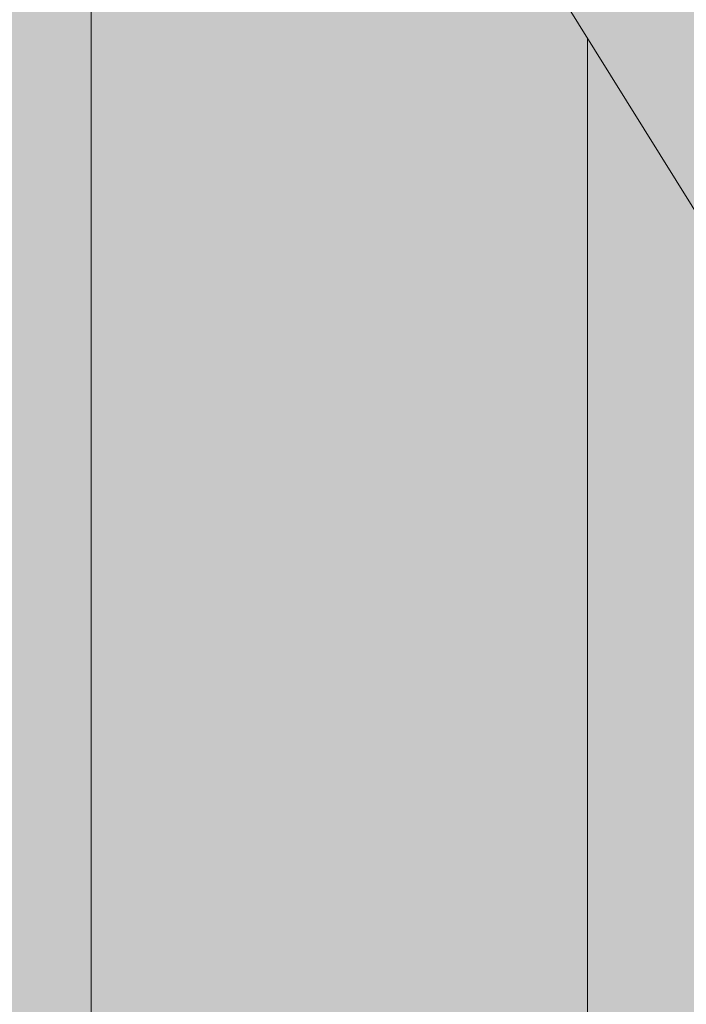
# Model space of a CAD drawing. Units: millimetres. Extents: x 11032 to 26788, y 3406 to 24505.
# Tile 48 of 78: x 15652 to 15719, y 16177 to 16276. Entities that reach past the tile are written whole.
import ezdxf

# ---------------------------------------------------------------- set-up
doc = ezdxf.new("R2010")
doc.units = ezdxf.units.MM
doc.header["$MEASUREMENT"] = 0
for name, color, linetype, lineweight in [('A-ANNO-DIMS', 2, 'Continuous', 18), ('A-GLAZ', 250, 'Continuous', 20), ('A-ROOF', 7, 'Continuous', 30), ('A-WALL', 7, 'Continuous', 35), ('E-LITE', 7, 'Continuous', 18), ('E-LITE-PATT', 7, 'Continuous', 13)]:
    doc.layers.add(name, color=color, linetype=linetype, lineweight=lineweight)
for name, color, linetype, lineweight, true_color in [('A-GLAZ-FRAM-PATT', 250, 'Continuous', 13, 0x262627), ('A-ROOF-PATT', 9, 'Continuous', 13, 0xc7c8ca), ('A-WALL-INTR-PATT', 251, 'Continuous', 13, 0x6c6b6a)]:
    doc.layers.add(name, color=color, linetype=linetype, lineweight=lineweight, true_color=true_color)
doc.styles.get("Standard").update_dxf_attribs({"font": 'arial.ttf'})
doc.dimstyles.get("Standard").update_dxf_attribs({"dimtxt": 150, "dimasz": 100, "dimexe": 10, "dimexo": 5, "dimgap": 5, "dimtad": 0, "dimtih": 1, "dimtoh": 1, "dimdec": 0, "dimzin": 0, "dimdsep": 46, "dimtxsty": 'Standard', "dimcen": 0.09, "dimadec": 0, "dimazin": 0, "dimtfac": 1, "dimtdec": 0, "dimtofl": 0, "dimtmove": 0, "dimatfit": 3, "dimfxl": 1, "dimtolj": 1, "dimtzin": 0, "dimarcsym": 0})

# ---------------------------------------------------------------- blocks, each defined once
blk = doc.blocks.new('*D36')
at = {"layer": 'A-ANNO-DIMS', "color": 0, "lineweight": -2, "transparency": 16777216}
for p, q in [((12301.265, 17115.885), (12301.265, 24416.858)), ((25397.404, 4466.399), (25397.404, 24416.858)), ((12401.265, 24406.858), (18569.198, 24406.858)), ((25297.404, 24406.858), (19129.471, 24406.858))]:
    blk.add_line(p, q, dxfattribs=at)
at = {"layer": 'A-ANNO-DIMS', "color": 0, "transparency": 16777216}
for points in [[(12401.265, 24423.525), (12401.265, 24390.191), (12301.265, 24406.858)], [(25297.404, 24423.525), (25297.404, 24390.191), (25397.404, 24406.858)]]:
    blk.add_solid(points, dxfattribs=at)
at = {"layer": 'Defpoints', "color": 0, "transparency": 16777216}
for p in [(25397.404, 24406.858), (12301.265, 17110.885), (25397.404, 4461.399)]:
    blk.add_point(p, dxfattribs=at)
at = {"layer": 'A-ANNO-DIMS', "color": 0, "transparency": 16777216, "insert": (18849.334, 24406.858), "char_height": 150, "attachment_point": 5}
blk.add_mtext('\\A1;13096', dxfattribs=at)
blk = doc.blocks.new('*D37')
at = {"layer": 'A-ANNO-DIMS', "color": 0, "lineweight": -2, "transparency": 16777216}
for p, q in [((18087.739, 23450.358), (11334.765, 23450.358)), ((11344.765, 23350.358), (11344.765, 14037.465)), ((11344.765, 4561.399), (11344.765, 13874.293)), ((12927.665, 4461.399), (11334.765, 4461.399))]:
    blk.add_line(p, q, dxfattribs=at)
at = {"layer": 'A-ANNO-DIMS', "color": 0, "transparency": 16777216}
for points in [[(11328.098, 23350.358), (11361.431, 23350.358), (11344.765, 23450.358)], [(11328.098, 4561.399), (11361.431, 4561.399), (11344.765, 4461.399)]]:
    blk.add_solid(points, dxfattribs=at)
at = {"layer": 'Defpoints', "color": 0, "transparency": 16777216}
for p in [(11344.765, 23450.358), (18092.739, 23450.358), (12932.665, 4461.399)]:
    blk.add_point(p, dxfattribs=at)
at = {"layer": 'A-ANNO-DIMS', "color": 0, "transparency": 16777216, "insert": (11344.765, 13955.879), "char_height": 150, "attachment_point": 5}
blk.add_mtext('\\A1;18989', dxfattribs=at)
blk = doc.blocks.new('*D45')
at = {"layer": 'A-ANNO-DIMS', "color": 0, "lineweight": -2, "transparency": 16777216}
for p, q in [((13792.367, 18518.925), (26363.904, 18518.925)), ((26353.904, 18418.925), (26353.904, 17450.319)), ((26353.904, 16318.44), (26353.904, 17287.045)), ((22902.404, 16218.44), (26363.904, 16218.44))]:
    blk.add_line(p, q, dxfattribs=at)
at = {"layer": 'A-ANNO-DIMS', "color": 0, "transparency": 16777216}
for points in [[(26337.237, 18418.925), (26370.57, 18418.925), (26353.904, 18518.925)], [(26337.237, 16318.44), (26370.57, 16318.44), (26353.904, 16218.44)]]:
    blk.add_solid(points, dxfattribs=at)
at = {"layer": 'Defpoints', "color": 0, "transparency": 16777216}
for p in [(13787.367, 18518.925), (26353.904, 18518.925), (22897.404, 16218.44)]:
    blk.add_point(p, dxfattribs=at)
at = {"layer": 'A-ANNO-DIMS', "color": 0, "transparency": 16777216, "insert": (26353.904, 17368.682), "char_height": 150, "attachment_point": 5}
blk.add_mtext('\\A1;2300.5', dxfattribs=at)
blk = doc.blocks.new('*D57')
at = {"layer": 'A-ANNO-DIMS', "color": 0, "lineweight": -2, "transparency": 16777216}
for p, q in [((14994.704, 7266.399), (14994.704, 24416.858)), ((20894.704, 7266.399), (20894.704, 24416.858)), ((15094.704, 24406.858), (17715.983, 24406.858)), ((20794.704, 24406.858), (18173.425, 24406.858))]:
    blk.add_line(p, q, dxfattribs=at)
at = {"layer": 'A-ANNO-DIMS', "color": 0, "transparency": 16777216}
for points in [[(15094.704, 24423.525), (15094.704, 24390.191), (14994.704, 24406.858)], [(20794.704, 24423.525), (20794.704, 24390.191), (20894.704, 24406.858)]]:
    blk.add_solid(points, dxfattribs=at)
at = {"layer": 'Defpoints', "color": 0, "transparency": 16777216}
for p in [(20894.704, 24406.858), (14994.704, 7261.399), (20894.704, 7261.399)]:
    blk.add_point(p, dxfattribs=at)
at = {"layer": 'A-ANNO-DIMS', "color": 0, "transparency": 16777216, "insert": (17944.704, 24406.858), "char_height": 150, "attachment_point": 5}
blk.add_mtext('\\A1;5900', dxfattribs=at)
blk = doc.blocks.new('*D60')
at = {"layer": 'A-ANNO-DIMS', "color": 0, "lineweight": -2, "transparency": 16777216}
for p, q in [((14994.704, 7266.399), (14994.704, 24416.858)), ((16344.704, 7266.399), (16344.704, 24416.858)), ((15094.704, 24406.858), (15448.043, 24406.858)), ((16244.704, 24406.858), (15891.365, 24406.858))]:
    blk.add_line(p, q, dxfattribs=at)
at = {"layer": 'A-ANNO-DIMS', "color": 0, "transparency": 16777216}
for points in [[(15094.704, 24423.525), (15094.704, 24390.191), (14994.704, 24406.858)], [(16244.704, 24423.525), (16244.704, 24390.191), (16344.704, 24406.858)]]:
    blk.add_solid(points, dxfattribs=at)
at = {"layer": 'Defpoints', "color": 0, "transparency": 16777216}
for p in [(16344.704, 24406.858), (14994.704, 7261.399), (16344.704, 7261.399)]:
    blk.add_point(p, dxfattribs=at)
at = {"layer": 'A-ANNO-DIMS', "color": 0, "transparency": 16777216, "insert": (15669.704, 24406.858), "char_height": 150, "attachment_point": 5}
blk.add_mtext('\\A1;1350', dxfattribs=at)

msp = doc.modelspace()

# ---------------------------------------------------------------- hatches: boundary and pattern name
at = {"layer": 'A-GLAZ-FRAM-PATT'}
h = msp.add_hatch(color=256, dxfattribs=at)
edge = h.paths.add_edge_path()
edge.add_line((15284.393, 17051.32), (15084.393, 17001.32))
edge.add_line((15084.393, 17001.32), (15084.393, 15951.32))
edge.add_spline(control_points=[(15084.393, 15951.32), (15157.266, 15924.219), (15224.458, 15897.808), (15284.393, 15870.289)], knot_values=[511.94901, 511.94901, 511.94901, 511.94901, 697.371598, 697.371598, 697.371598, 697.371598], degree=3, periodic=0)
edge.add_line((15284.393, 15870.289), (15284.393, 17051.32))
edge = h.paths.add_edge_path()
edge.add_line((15659.393, 16354.387), (15459.393, 16675.629))
edge.add_line((15459.393, 16675.629), (15459.393, 15771.505))
edge.add_spline(control_points=[(15459.393, 15771.505), (15501.891, 15741.568), (15571.096, 15682.692), (15632.72, 15612.509), (15659.393, 15578.299)], knot_values=[905.064582, 905.064582, 905.064582, 905.064582, 1079.468271, 1223.158435, 1223.158435, 1223.158435, 1223.158435], degree=3, periodic=0)
edge.add_line((15659.393, 15578.299), (15659.393, 16354.387))
h.paths.add_polyline_path([(15284.393, 17051.32), (15284.393, 16956.717), (15784.393, 16153.61), (15784.393, 16248.213)])
h = msp.add_hatch(color=256, dxfattribs=at)
edge = h.paths.add_edge_path()
edge.add_spline(control_points=[(15409.393, 16728.446), (15384.197, 16718.122), (15359.177, 16707.259), (15334.393, 16695.842)], knot_values=[2052.671403, 2052.671403, 2052.671403, 2052.671403, 2131.020164, 2131.020164, 2131.020164, 2131.020164], degree=3, periodic=0)
edge.add_line((15334.393, 16695.842), (15334.393, 15846.165))
edge.add_spline(control_points=[(15334.393, 15846.165), (15360.99, 15832.635), (15385.89, 15818.741), (15409.393, 15804.345)], knot_values=[750.83835, 750.83835, 750.83835, 750.83835, 839.475874, 839.475874, 839.475874, 839.475874], degree=3, periodic=0)
edge.add_line((15409.393, 15804.345), (15409.393, 16728.446))
edge = h.paths.add_edge_path()
edge.add_line((15784.393, 16153.61), (15709.393, 16274.076))
edge.add_line((15709.393, 16274.076), (15709.393, 15509.31))
edge.add_spline(control_points=[(15709.393, 15509.31), (15712.398, 15504.862), (15738.373, 15465.922), (15763.422, 15424.165), (15784.393, 15385.996)], knot_values=[1315.342429, 1315.342429, 1315.342429, 1315.342429, 1332.382415, 1463.285048, 1463.285048, 1463.285048, 1463.285048], degree=3, periodic=0)
edge.add_line((15784.393, 15385.996), (15784.393, 16153.61))
at = {"layer": 'A-ROOF-PATT'}
h = msp.add_hatch(color=256, dxfattribs=at)
edge = h.paths.add_edge_path()
edge.add_spline(control_points=[(17532.827, 17324.837), (17391.335, 17349.016), (16840.872, 17494.912), (16080.055, 18069.544), (14738.803, 18299.641), (13382.429, 18838.336), (12580.532, 17870.207), (12430.422, 17563.822)], knot_values=[2977.602794, 2977.602794, 2977.602794, 2977.602794, 3438.18406, 4811.646302, 5622.867548, 7588.028819, 8560.668579, 8560.668579, 8560.668579, 8560.668579], degree=3, periodic=0)
edge.add_spline(control_points=[(12430.422, 17563.822), (12437.904, 17573.36), (12445.386, 17582.899), (12452.869, 17592.437), (12452.869, 17592.438), (12452.869, 17592.438), (12452.869, 17592.438)], knot_values=[1408.564138, 1408.564138, 1408.564138, 1408.564138, 1444.85989, 1444.85989, 1444.85989, 1444.860118, 1444.860118, 1444.860118, 1444.860118], degree=3, periodic=0)
edge.add_spline(control_points=[(12452.869, 17592.438), (12555.432, 17723.185), (12736.557, 17929.686), (13044.86, 18114.643), (13219.943, 18189.644), (13299.92, 18220.646)], knot_values=[339.318246, 339.318246, 339.318246, 339.318246, 836.834997, 1151.251293, 1408.564138, 1408.564138, 1408.564138, 1408.564138], degree=3, periodic=0)
edge.add_spline(control_points=[(13299.92, 18220.646), (13299.998, 18220.689), (13300.077, 18220.732), (13319.738, 18231.488), (13339.24, 18241.402), (13388.645, 18264.703), (13418.466, 18277.069), (13478.019, 18298.648), (13507.751, 18307.861), (13544.561, 18317.488), (13551.584, 18319.245), (13558.612, 18320.924)], knot_values=[3783.895097, 3783.895097, 3783.895097, 3783.895097, 3784.17371, 3784.17371, 3853.466675, 3853.466675, 3960.240192, 3960.240192, 4067.013709, 4067.013709, 4092.174465, 4092.174465, 4092.174465, 4092.174465], degree=3, periodic=0)
edge.add_spline(control_points=[(13558.612, 18320.924), (13581.407, 18326.373), (13604.25, 18331.007), (13657.184, 18339.957), (13687.338, 18343.732), (13748.098, 18348.892), (13778.704, 18350.276), (13840.46, 18350.833), (13871.609, 18350.005), (13934.496, 18346.313), (13966.232, 18343.449), (14030.297, 18335.871), (14062.625, 18331.158), (14127.853, 18320.088), (14160.753, 18313.73), (14241.357, 18296.556), (14289.343, 18284.997), (14386.31, 18259.688), (14435.291, 18245.941), (14534.161, 18217.034), (14584.049, 18201.875), (14684.682, 18170.964), (14735.427, 18155.212), (14837.763, 18123.971), (14889.354, 18108.482), (14954.971, 18089.677), (14968.586, 18085.823), (14992.391, 18079.184), (15002.566, 18076.376), (15021.739, 18071.153), (15030.731, 18068.729), (15047.707, 18064.21), (15055.694, 18062.106), (15079.815, 18055.825), (15095.905, 18051.728), (15143.966, 18039.717), (15175.729, 18032.084), (15254.84, 18013.501), (15301.798, 18002.866), (15394.186, 17981.845), (15439.615, 17971.459), (15528.833, 17950.135), (15572.62, 17939.197), (15658.477, 17916.021), (15700.546, 17903.785), (15753.633, 17886.734), (15765.446, 17882.835), (15786.574, 17875.653), (15795.915, 17872.404), (15810.108, 17867.349), (15814.99, 17865.588), (15824.736, 17862.029), (15829.611, 17860.226), (15844.241, 17854.75), (15854.002, 17851.008), (15883.312, 17839.521), (15902.885, 17831.512), (15966.355, 17804.548), (16010.39, 17784.302), (16098.838, 17741.267), (16143.25, 17718.478), (16232.497, 17671.098), (16277.332, 17646.507), (16367.515, 17596.295), (16412.862, 17570.676), (16504.202, 17519.209), (16550.194, 17493.362), (16643.009, 17442.263), (16689.831, 17417.011), (16756.517, 17382.472), (16775.937, 17372.58), (16795.455, 17362.84)], knot_values=[4092.174465, 4092.174465, 4092.174465, 4092.174465, 4173.787226, 4173.787226, 4280.560743, 4280.560743, 4387.33426, 4387.33426, 4494.107777, 4494.107777, 4600.881294, 4600.881294, 4707.654811, 4707.654811, 4814.428328, 4814.428328, 4967.12624, 4967.12624, 5119.824153, 5119.824153, 5272.522066, 5272.522066, 5425.219978, 5425.219978, 5577.917891, 5577.917891, 5617.785332, 5617.785332, 5647.464848, 5647.464848, 5673.611025, 5673.611025, 5696.747607, 5696.747607, 5743.68189, 5743.68189, 5837.550457, 5837.550457, 5979.726105, 5979.726105, 6121.901752, 6121.901752, 6264.0774, 6264.0774, 6406.253047, 6406.253047, 6447.258585, 6447.258585, 6480.042088, 6480.042088, 6497.307706, 6497.307706, 6514.573324, 6514.573324, 6549.10456, 6549.10456, 6618.167032, 6618.167032, 6772.661017, 6772.661017, 6927.155002, 6927.155002, 7081.648987, 7081.648987, 7236.142972, 7236.142972, 7390.636957, 7390.636957, 7545.130942, 7545.130942, 7608.199287, 7608.199287, 7608.199287, 7608.199287], degree=3, periodic=0)
edge.add_spline(control_points=[(16795.455, 17362.84), (16814.335, 17349.456), (16832.897, 17336.263), (16873.225, 17307.197), (16894.778, 17291.386), (16936.221, 17259.941), (16956.11, 17244.308), (16993.863, 17213.094), (17011.726, 17197.514), (17041.993, 17169.265), (17054.791, 17156.601), (17078.762, 17131.225), (17089.933, 17118.516), (17110.618, 17092.991), (17120.131, 17080.178), (17130.17, 17065.264), (17131.487, 17063.277), (17133.77, 17059.776), (17134.746, 17058.261), (17136.69, 17055.205), (17137.657, 17053.668), (17140.539, 17049.025), (17142.438, 17045.89), (17148.068, 17036.367), (17151.732, 17029.859), (17163.03, 17008.788), (17170.335, 16993.646), (17184.087, 16961.978), (17190.534, 16945.453), (17202.562, 16911.165), (17208.142, 16893.402), (17218.448, 16856.821), (17223.173, 16838.003), (17231.801, 16799.51), (17235.705, 16779.837), (17241.533, 16746.739), (17243.676, 16733.5), (17247.718, 16706.37), (17249.608, 16692.472), (17252.066, 16672.69), (17252.761, 16666.875), (17254.1, 16655.226), (17254.744, 16649.4), (17256.596, 16631.917), (17257.727, 16620.254), (17260.823, 16585.238), (17262.489, 16561.858), (17266.551, 16488.654), (17267.658, 16438.661), (17267.349, 16375.228), (17267.193, 16362.07), (17266.95, 16348.891)], knot_values=[15.113047, 15.113047, 15.113047, 15.113047, 82.699515, 82.699515, 165.399029, 165.399029, 248.098544, 248.098544, 330.798058, 330.798058, 397.941946, 397.941946, 465.085833, 465.085833, 532.229721, 532.229721, 542.533741, 542.533741, 550.356816, 550.356816, 558.179891, 558.179891, 573.82604, 573.82604, 605.118339, 605.118339, 672.764061, 672.764061, 740.409783, 740.409783, 808.055505, 808.055505, 875.701227, 875.701227, 943.346949, 943.346949, 987.661349, 987.661349, 1033.412161, 1033.412161, 1052.385088, 1052.385088, 1071.358014, 1071.358014, 1109.303867, 1109.303867, 1185.195572, 1185.195572, 1346.441903, 1346.441903, 1388.558663, 1388.558663, 1388.558663, 1388.558663], degree=3, periodic=0)
edge.add_spline(control_points=[(17266.95, 16348.891), (17266.95, 16348.891), (17266.95, 16348.891), (17266.95, 16348.891), (17253.182, 15602.417), (17239.414, 14855.943), (17225.646, 14109.469)], knot_values=[1388.558663, 1388.558663, 1388.558663, 1388.558663, 1388.558965, 1388.558965, 1388.558965, 3774.076766, 3774.076766, 3774.076766, 3774.076766], degree=3, periodic=0)
edge.add_spline(control_points=[(17225.646, 14109.469), (17226.198, 14109.827), (17226.748, 14110.185), (17242.065, 14120.191), (17255.956, 14130.116), (17274.422, 14144.286), (17279.609, 14148.386), (17284.686, 14152.511)], knot_values=[1926.342397, 1926.342397, 1926.342397, 1926.342397, 1927.316729, 1927.316729, 1953.512176, 1953.512176, 1964.073235, 1964.073235, 1964.073235, 1964.073235], degree=3, periodic=0)
edge.add_spline(control_points=[(17284.686, 14152.511), (17315.791, 14194.761), (17384.413, 14446.273), (17407.128, 14793.401), (17407.093, 15295.84), (17423.274, 15626.362), (17415.601, 15782.507)], knot_values=[0, 0, 0, 0, 163.255467, 619.229677, 1171.862448, 1621.635556, 1621.635556, 1621.635556, 1621.635556], degree=3, periodic=0)
edge.add_spline(control_points=[(17415.601, 15782.507), (17438.21, 16077.57), (17410.495, 16533.484), (17390.893, 17030.649), (17301.082, 17169.349)], knot_values=[543.978475, 543.978475, 543.978475, 543.978475, 1452.985277, 1960.011493, 1960.011493, 1960.011493, 1960.011493], degree=3, periodic=0)
edge.add_spline(control_points=[(17301.082, 17169.349), (17346.58, 17157.64), (17392.235, 17147.336), (17467.161, 17132.609), (17496.336, 17127.412), (17525.58, 17122.709)], knot_values=[8131.593939, 8131.593939, 8131.593939, 8131.593939, 8269.734927, 8269.734927, 8357.501665, 8357.501665, 8357.501665, 8357.501665], degree=3, periodic=0)
edge.add_line((17525.58, 17122.709), (17532.827, 17324.837))
edge = h.paths.add_edge_path(flags=17)
edge.add_spline(control_points=[(13340.537, 14602.706), (13316.172, 14726.456), (13323.666, 14932.342), (13637.836, 15081.117), (13863.248, 15171.051), (14002.1, 15224.503), (14058.539, 15244.876)], knot_values=[680.893186, 680.893186, 680.893186, 680.893186, 1033.472829, 1337.400833, 1604.721426, 1784.294472, 1784.294472, 1784.294472, 1784.294472], degree=3, periodic=0)
edge.add_spline(control_points=[(14058.539, 15244.876), (14058.289, 15275.236), (14057.634, 15305.434), (14055.312, 15376.527), (14053.359, 15417.248), (14048.642, 15497.048), (14045.89, 15536.143), (14042.888, 15574.619)], knot_values=[6573.106542, 6573.106542, 6573.106542, 6573.106542, 6636.733001, 6636.733001, 6723.889055, 6723.889055, 6809.632877, 6809.632877, 6809.632877, 6809.632877], degree=3, periodic=0)
edge.add_spline(control_points=[(14042.888, 15574.619), (13546.54, 15403.221), (13074.735, 15143.241), (13277.36, 14695.339), (13340.537, 14602.706)], knot_values=[503.792578, 503.792578, 503.792578, 503.792578, 1728.178761, 2051.34844, 2051.34844, 2051.34844, 2051.34844], degree=3, periodic=0)
h = msp.add_hatch(color=256, dxfattribs=at)
h.set_gradient(color1=(254, 234, 185), color2=(254, 204, 102), name='HEMISPHERICAL')
edge = h.paths.add_edge_path()
edge.add_line((15084.393, 17001.32), (15284.393, 17051.32))
edge.add_line((15284.393, 17051.32), (15470.537, 16752.334))
edge.add_spline(control_points=[(15470.537, 16752.334), (15683.311, 16831.508), (16106.827, 16912.335), (16625.609, 16876.997), (17083.498, 16357.78), (17257.801, 16180.113)], knot_values=[0, 0, 0, 0, 655.293633, 1252.015784, 1989.616286, 1989.616286, 1989.616286, 1989.616286], degree=3, periodic=0)
edge.add_spline(control_points=[(17257.801, 16180.113), (17260.851, 16236.372), (17263.9, 16292.632), (17266.95, 16348.891)], knot_values=[1132.996772, 1132.996772, 1132.996772, 1132.996772, 1198.046422, 1198.046422, 1198.046422, 1198.046422], degree=3, periodic=0)
edge.add_spline(control_points=[(17266.95, 16348.891), (17267.193, 16362.07), (17267.349, 16375.228), (17267.658, 16438.661), (17266.551, 16488.654), (17262.489, 16561.858), (17260.823, 16585.238), (17257.727, 16620.254), (17256.596, 16631.917), (17254.744, 16649.4), (17254.1, 16655.226), (17252.761, 16666.875), (17252.066, 16672.69), (17249.608, 16692.472), (17247.718, 16706.37), (17243.676, 16733.5), (17241.533, 16746.739), (17235.705, 16779.837), (17231.801, 16799.51), (17223.173, 16838.003), (17218.448, 16856.821), (17208.142, 16893.402), (17202.562, 16911.165), (17190.534, 16945.453), (17184.087, 16961.978), (17170.335, 16993.646), (17163.03, 17008.788), (17151.732, 17029.859), (17148.068, 17036.367), (17142.438, 17045.89), (17140.539, 17049.025), (17137.657, 17053.668), (17136.69, 17055.205), (17134.746, 17058.261), (17133.77, 17059.776), (17131.487, 17063.277), (17130.17, 17065.264), (17120.131, 17080.178), (17110.618, 17092.991), (17089.933, 17118.516), (17078.762, 17131.225), (17054.791, 17156.601), (17041.993, 17169.265), (17011.726, 17197.514), (16993.863, 17213.094), (16956.11, 17244.308), (16936.221, 17259.941), (16894.778, 17291.386), (16873.225, 17307.197), (16832.897, 17336.263), (16814.335, 17349.456), (16795.455, 17362.84)], knot_values=[15.113047, 15.113047, 15.113047, 15.113047, 57.229808, 57.229808, 218.476138, 218.476138, 294.367844, 294.367844, 332.313696, 332.313696, 351.286623, 351.286623, 370.259549, 370.259549, 416.010361, 416.010361, 460.324761, 460.324761, 527.970483, 527.970483, 595.616205, 595.616205, 663.261927, 663.261927, 730.907649, 730.907649, 798.553371, 798.553371, 829.84567, 829.84567, 845.49182, 845.49182, 853.314895, 853.314895, 861.137969, 861.137969, 871.441989, 871.441989, 938.585877, 938.585877, 1005.729765, 1005.729765, 1072.873652, 1072.873652, 1155.573167, 1155.573167, 1238.272681, 1238.272681, 1320.972196, 1320.972196, 1388.558663, 1388.558663, 1388.558663, 1388.558663], degree=3, periodic=0)
edge.add_spline(control_points=[(16795.455, 17362.84), (16775.937, 17372.58), (16756.517, 17382.472), (16689.831, 17417.011), (16643.009, 17442.263), (16550.194, 17493.362), (16504.202, 17519.209), (16412.862, 17570.676), (16367.515, 17596.295), (16277.332, 17646.507), (16232.497, 17671.098), (16143.25, 17718.478), (16098.838, 17741.267), (16010.39, 17784.302), (15966.355, 17804.548), (15902.885, 17831.512), (15883.312, 17839.521), (15854.002, 17851.008), (15844.241, 17854.75), (15829.611, 17860.226), (15824.736, 17862.029), (15814.99, 17865.588), (15810.108, 17867.349), (15795.915, 17872.404), (15786.574, 17875.653), (15765.446, 17882.835), (15753.633, 17886.734), (15700.546, 17903.785), (15658.477, 17916.021), (15572.62, 17939.197), (15528.833, 17950.135), (15439.615, 17971.459), (15394.186, 17981.845), (15301.798, 18002.866), (15254.84, 18013.501), (15175.729, 18032.084), (15143.966, 18039.717), (15095.905, 18051.728), (15079.815, 18055.825), (15055.694, 18062.106), (15047.707, 18064.21), (15030.731, 18068.729), (15021.739, 18071.153), (15002.566, 18076.376), (14992.391, 18079.184), (14968.586, 18085.823), (14954.971, 18089.677), (14889.354, 18108.482), (14837.763, 18123.971), (14735.427, 18155.212), (14684.682, 18170.964), (14584.049, 18201.875), (14534.161, 18217.034), (14435.291, 18245.941), (14386.31, 18259.688), (14289.343, 18284.997), (14241.357, 18296.556), (14160.753, 18313.73), (14127.853, 18320.088), (14062.625, 18331.158), (14030.297, 18335.871), (13966.232, 18343.449), (13934.496, 18346.313), (13871.609, 18350.005), (13840.46, 18350.833), (13778.704, 18350.276), (13748.098, 18348.892), (13687.338, 18343.732), (13657.184, 18339.957), (13604.25, 18331.007), (13581.407, 18326.373), (13558.612, 18320.924)], knot_values=[4092.174465, 4092.174465, 4092.174465, 4092.174465, 4155.24281, 4155.24281, 4309.736795, 4309.736795, 4464.23078, 4464.23078, 4618.724765, 4618.724765, 4773.21875, 4773.21875, 4927.712735, 4927.712735, 5082.20672, 5082.20672, 5151.269192, 5151.269192, 5185.800428, 5185.800428, 5203.066045, 5203.066045, 5220.331663, 5220.331663, 5253.115167, 5253.115167, 5294.120705, 5294.120705, 5436.296352, 5436.296352, 5578.472, 5578.472, 5720.647647, 5720.647647, 5862.823295, 5862.823295, 5956.691861, 5956.691861, 6003.626145, 6003.626145, 6026.762727, 6026.762727, 6052.908904, 6052.908904, 6082.58842, 6082.58842, 6122.455861, 6122.455861, 6275.153773, 6275.153773, 6427.851686, 6427.851686, 6580.549599, 6580.549599, 6733.247511, 6733.247511, 6885.945424, 6885.945424, 6992.718941, 6992.718941, 7099.492458, 7099.492458, 7206.265975, 7206.265975, 7313.039492, 7313.039492, 7419.813009, 7419.813009, 7526.586526, 7526.586526, 7608.199287, 7608.199287, 7608.199287, 7608.199287], degree=3, periodic=0)
edge.add_spline(control_points=[(13558.612, 18320.924), (13472.381, 18287.498), (13386.15, 18254.072), (13299.92, 18220.646), (13299.92, 18220.646), (13299.92, 18220.646), (13299.92, 18220.646)], knot_values=[61.883246, 61.883246, 61.883246, 61.883246, 339.317975, 339.317975, 339.317975, 339.318246, 339.318246, 339.318246, 339.318246], degree=3, periodic=0)
edge.add_spline(control_points=[(13299.92, 18220.646), (13219.943, 18189.644), (13044.86, 18114.643), (12736.557, 17929.686), (12555.432, 17723.185), (12452.869, 17592.438)], knot_values=[339.318246, 339.318246, 339.318246, 339.318246, 596.631091, 911.047387, 1408.564138, 1408.564138, 1408.564138, 1408.564138], degree=3, periodic=0)
edge.add_spline(control_points=[(12452.869, 17592.438), (12452.869, 17592.438), (12452.869, 17592.438), (12452.869, 17592.437), (12445.386, 17582.899), (12437.904, 17573.36), (12430.422, 17563.822)], knot_values=[1408.564138, 1408.564138, 1408.564138, 1408.564138, 1408.564366, 1408.564366, 1408.564366, 1444.860118, 1444.860118, 1444.860118, 1444.860118], degree=3, periodic=0)
edge.add_spline(control_points=[(12430.422, 17563.822), (12373.797, 17448.248), (12157.302, 16836.764), (12751.985, 16393.69), (13424.325, 15907.903), (14042.888, 15574.619)], knot_values=[0, 0, 0, 0, 366.899303, 1975.594108, 2977.602794, 2977.602794, 2977.602794, 2977.602794], degree=3, periodic=0)
edge.add_spline(control_points=[(14042.888, 15574.619), (14042.839, 15575.252), (14042.789, 15575.886), (14039.681, 15615.607), (14036.366, 15654.052), (14029.551, 15729.305), (14026.05, 15766.114), (14019.175, 15837.686), (14015.8, 15872.45), (13903.823, 16338.596)], knot_values=[6310.22615, 6310.22615, 6310.22615, 6310.22615, 6311.638381, 6311.638381, 6398.794435, 6398.794435, 6485.950488, 6485.950488, 6573.106542, 6573.106542, 6573.106542, 6573.106542], degree=3, periodic=0)
edge.add_spline(control_points=[(13903.823, 16338.596), (14237.315, 16236.889), (14456.623, 16167.555), (14614.196, 16115.84)], knot_values=[0, 0, 0, 0, 202.985342, 202.985342, 202.985342, 202.985342], degree=3, periodic=0)
edge.add_spline(control_points=[(14614.196, 16115.84), (14663.209, 16178.992), (14799.965, 16341.237), (14969.915, 16481.426), (15084.393, 16556.825)], knot_values=[2405.034504, 2405.034504, 2405.034504, 2405.034504, 2644.882697, 3039.270727, 3039.270727, 3039.270727, 3039.270727], degree=3, periodic=0)
edge.add_line((15084.393, 16556.825), (15084.393, 17001.32))
h.paths.add_polyline_path([(14195.599, 17606.181, -1), (14395.599, 17606.181, -1)], flags=16)
h.paths.add_polyline_path([(13310.178, 17032.97, -1), (13510.178, 17032.97, -1)], flags=16)
h = msp.add_hatch(color=256, dxfattribs=at)
h.set_gradient(color1=(254, 234, 185), color2=(254, 204, 102), name='HEMISPHERICAL')
edge = h.paths.add_edge_path()
edge.add_spline(control_points=[(16560.042, 14907.752), (16569.192, 14907.664), (16578.343, 14907.575), (16587.493, 14907.486), (16832.101, 14905.115), (17122.895, 14902.296), (16849.359, 14976.117), (16870.954, 15304.114), (17098.337, 15241.178), (17235.385, 15203.245)], knot_values=[0, 0, 0, 0, 14.867439, 14.867439, 14.867439, 412.294309, 487.334592, 708.6416, 1044.393945, 1044.393945, 1044.393945, 1044.393945], degree=3, periodic=0)
edge.add_line((16587.504, 14907.486), (16560.207, 14907.486))
edge.add_line((16560.207, 14907.486), (15784.393, 16153.61))
edge.add_line((15784.393, 16153.61), (15784.393, 15385.996))
edge.add_spline(control_points=[(15784.393, 15385.996), (15798.391, 15360.52), (15847.198, 15266.214), (15887.196, 15168.614), (15912.903, 15096.727)], knot_values=[1463.285048, 1463.285048, 1463.285048, 1463.285048, 1550.659771, 1779.959936, 1779.959936, 1779.959936, 1779.959936], degree=3, periodic=0)
edge.add_spline(control_points=[(15912.903, 15096.727), (15913.652, 15095.649), (15914.403, 15094.565), (15925.191, 15078.948), (15935.516, 15063.47), (15956.582, 15030.918), (15967.324, 15013.844), (15989.119, 14978.386), (16000.173, 14960.003), (16022.525, 14922.193), (16033.824, 14902.767), (16056.63, 14863.116), (16068.138, 14842.891), (16091.349, 14801.871), (16103.053, 14781.075), (16126.666, 14739.118), (16138.575, 14717.958), (16162.628, 14675.459), (16174.772, 14654.12), (16199.352, 14611.428), (16211.787, 14590.075), (16237.037, 14547.491), (16249.851, 14526.26), (16271.946, 14490.566), (16281.092, 14476.044), (16299.694, 14447.129), (16309.149, 14432.737), (16328.456, 14404.098), (16338.307, 14389.85), (16358.518, 14361.503), (16368.879, 14347.403), (16390.266, 14319.347), (16401.291, 14305.391), (16420.626, 14281.969), (16428.703, 14272.467), (16445.363, 14253.527), (16453.946, 14244.088), (16471.727, 14225.278), (16480.926, 14215.907), (16500.075, 14197.247), (16510.026, 14187.959), (16530.844, 14169.504), (16541.71, 14160.337), (16564.549, 14142.195), (16576.522, 14133.22), (16597.69, 14118.448), (16606.528, 14112.565), (16624.87, 14101.004), (16634.376, 14095.326), (16654.117, 14084.255), (16664.352, 14078.862), (16685.603, 14068.46), (16696.619, 14063.452), (16719.46, 14053.944), (16731.285, 14049.444), (16755.742, 14041.097), (16768.374, 14037.251), (16794.396, 14030.368), (16807.787, 14027.332), (16835.229, 14022.23), (16849.279, 14020.163), (16877.882, 14017.141), (16892.435, 14016.186), (16921.835, 14015.489), (16936.683, 14015.749), (16961.564, 14017.241), (16971.582, 14018.127), (16986.57, 14019.883), (16991.56, 14020.54), (16999.027, 14021.63), (17001.514, 14022.011), (17006.48, 14022.809), (17008.962, 14023.225), (17014.824, 14024.251), (17018.193, 14024.875), (17036.262, 14028.398), (17050.55, 14031.826), (17078.171, 14039.583), (17091.505, 14043.912), (17115.643, 14052.705), (17126.557, 14057.089), (17137.108, 14061.688)], knot_values=[2010.763962, 2010.763962, 2010.763962, 2010.763962, 2014.702983, 2014.702983, 2067.238337, 2067.238337, 2119.773691, 2119.773691, 2172.309046, 2172.309046, 2224.8444, 2224.8444, 2277.379754, 2277.379754, 2329.915109, 2329.915109, 2382.450463, 2382.450463, 2434.985817, 2434.985817, 2487.521172, 2487.521172, 2540.056526, 2540.056526, 2576.317929, 2576.317929, 2612.579332, 2612.579332, 2648.840735, 2648.840735, 2685.102138, 2685.102138, 2721.363541, 2721.363541, 2746.252015, 2746.252015, 2771.14049, 2771.14049, 2796.028964, 2796.028964, 2820.917439, 2820.917439, 2845.805913, 2845.805913, 2870.694388, 2870.694388, 2887.513276, 2887.513276, 2904.332164, 2904.332164, 2921.151052, 2921.151052, 2937.96994, 2937.96994, 2954.788828, 2954.788828, 2971.607717, 2971.607717, 2988.426605, 2988.426605, 3005.245493, 3005.245493, 3022.064381, 3022.064381, 3038.883269, 3038.883269, 3050.197545, 3050.197545, 3055.854683, 3055.854683, 3058.683252, 3058.683252, 3061.511821, 3061.511821, 3065.393417, 3065.393417, 3082.466872, 3082.466872, 3099.540326, 3099.540326, 3114.543344, 3114.543344, 3114.543344, 3114.543344], degree=3, periodic=0)
edge.add_spline(control_points=[(17137.108, 14061.688), (17165.253, 14274.398), (17209.97, 14653.885), (17230.2, 15035.586), (17235.385, 15203.245)], knot_values=[1968.080456, 1968.080456, 1968.080456, 1968.080456, 2611.528287, 3114.537926, 3114.537926, 3114.537926, 3114.537926], degree=3, periodic=0)
edge = h.paths.add_edge_path()
edge.add_spline(control_points=[(16856.103, 14956.992), (16852.841, 14961.219), (16849.83, 14965.576), (16842.539, 14977.287), (16838.658, 14984.798), (16832.033, 15000.109), (16829.289, 15007.911), (16824.126, 15026.008), (16822.047, 15036.354), (16819.308, 15057.097), (16818.649, 15067.496), (16818.576, 15088.188), (16819.162, 15098.483), (16821.467, 15118.823), (16823.186, 15128.868), (16827.696, 15148.567), (16830.486, 15158.22), (16836.065, 15173.969), (16838.565, 15180.211), (16844.079, 15192.402), (16847.092, 15198.353), (16852.029, 15207.021), (16853.744, 15209.868), (16857.321, 15215.468), (16859.188, 15218.226), (16863.017, 15223.558), (16864.978, 15226.136), (16872.565, 15235.558), (16878.593, 15241.952), (16891.428, 15253.591), (16898.232, 15258.834), (16912.397, 15268.127), (16919.756, 15272.176), (16934.816, 15279.138), (16942.515, 15282.052), (16958.1, 15286.873), (16965.985, 15288.78), (16984.013, 15292.142), (16994.186, 15293.334), (17014.631, 15294.619), (17024.904, 15294.713), (17048.453, 15293.935), (17061.76, 15292.783), (17088.519, 15289.422), (17101.972, 15287.211), (17131.961, 15281.46), (17148.526, 15277.734), (17181.692, 15269.627), (17198.292, 15265.245), (17222.182, 15258.759), (17229.535, 15256.737), (17236.862, 15254.714)], knot_values=[9.663953, 9.663953, 9.663953, 9.663953, 20.035167, 20.035167, 36.941175, 36.941175, 53.847184, 53.847184, 75.779569, 75.779569, 97.711954, 97.711954, 119.644339, 119.644339, 141.576724, 141.576724, 163.509109, 163.509109, 178.382995, 178.382995, 193.25688, 193.25688, 200.693823, 200.693823, 208.130766, 208.130766, 215.444859, 215.444859, 235.579592, 235.579592, 255.714326, 255.714326, 275.84906, 275.84906, 295.983794, 295.983794, 316.118527, 316.118527, 341.722054, 341.722054, 367.325581, 367.325581, 400.157243, 400.157243, 432.988905, 432.988905, 473.044017, 473.044017, 513.099128, 513.099128, 530.9693, 530.9693, 530.9693, 530.9693], degree=3, periodic=0)
edge.add_spline(control_points=[(17236.862, 15254.714), (17240.377, 15387.456), (17242.496, 15609.536), (17239.752, 15831.567), (17250.544, 16044.717)], knot_values=[1250.981862, 1250.981862, 1250.981862, 1250.981862, 1649.151658, 1916.613987, 1916.613987, 1916.613987, 1916.613987], degree=3, periodic=0)
edge.add_spline(control_points=[(17250.544, 16044.717), (17229.169, 16066.505), (17207.794, 16088.292), (17186.419, 16110.08), (17186.418, 16110.08), (17186.418, 16110.081), (17186.418, 16110.081)], knot_values=[-88.518558, -88.518558, -88.518558, -88.518558, -0.001278, -0.001278, -0.001278, 0, 0, 0, 0], degree=3, periodic=0)
edge.add_spline(control_points=[(17186.418, 16110.081), (17169.261, 16127.569), (17151.499, 16145.947), (17114.892, 16184.084), (17096.046, 16203.842), (17057.437, 16244.305), (17037.673, 16265.01), (16997.415, 16306.918), (16976.921, 16328.12), (16927.79, 16378.347), (16898.924, 16407.388), (16840.771, 16464.327), (16811.484, 16492.225), (16758.449, 16540.764), (16734.666, 16561.798), (16687.634, 16601.588), (16664.382, 16620.344), (16624.116, 16650.909), (16606.897, 16663.324), (16583.769, 16678.999), (16577.49, 16683.149), (16567.144, 16689.805), (16563.039, 16692.397), (16550.823, 16699.959), (16542.775, 16704.739), (16526.841, 16713.814), (16518.956, 16718.108), (16495.524, 16730.301), (16480.199, 16737.514), (16449.97, 16750.334), (16435.066, 16755.942), (16405.476, 16765.764), (16390.79, 16769.979), (16361.418, 16777.195), (16346.731, 16780.197), (16317.147, 16785.133), (16302.249, 16787.067), (16272.053, 16789.992), (16256.756, 16790.981), (16225.609, 16792.125), (16209.759, 16792.279), (16177.385, 16791.865), (16160.862, 16791.296), (16136.98, 16790.07), (16129.942, 16789.661), (16118.22, 16788.91), (16113.574, 16788.594), (16103.645, 16787.886), (16098.362, 16787.489), (16087.761, 16786.652), (16082.439, 16786.212), (16066.413, 16784.825), (16055.649, 16783.812), (16023.135, 16780.505), (16001.164, 16777.942), (15934.539, 16769.141), (15889.17, 16761.791), (15797.417, 16743.949), (15751.033, 16733.457), (15645.217, 16705.796), (15585.74, 16687.58), (15526.207, 16666.217), (15525.367, 16665.915), (15524.528, 16665.613)], knot_values=[0, 0, 0, 0, 71.050145, 71.050145, 142.100291, 142.100291, 213.150436, 213.150436, 284.200582, 284.200582, 381.323193, 381.323193, 478.445804, 478.445804, 557.821985, 557.821985, 637.198165, 637.198165, 698.312259, 698.312259, 721.397137, 721.397137, 736.779089, 736.779089, 767.542992, 767.542992, 798.306896, 798.306896, 859.834702, 859.834702, 921.362509, 921.362509, 982.890315, 982.890315, 1044.418122, 1044.418122, 1105.945928, 1105.945928, 1167.473735, 1167.473735, 1229.001542, 1229.001542, 1290.529348, 1290.529348, 1315.899004, 1315.899004, 1332.381279, 1332.381279, 1350.905266, 1350.905266, 1369.429252, 1369.429252, 1406.477225, 1406.477225, 1480.573171, 1480.573171, 1628.765063, 1628.765063, 1776.956955, 1776.956955, 1966.310925, 1966.310925, 1969.019495, 1969.019495, 1969.019495, 1969.019495], degree=3, periodic=0)
edge.add_line((15524.528, 16665.613), (16587.978, 14957.484))
edge.add_spline(control_points=[(16587.978, 14957.484), (16605.253, 14957.316), (16622.516, 14957.149), (16665.945, 14956.759), (16691.933, 14956.554), (16742.419, 14956.302), (16766.918, 14956.255), (16813.531, 14956.412), (16835.647, 14956.617), (16856.103, 14956.992)], knot_values=[872.218193, 872.218193, 872.218193, 872.218193, 900.28573, 900.28573, 943.365989, 943.365989, 986.446248, 986.446248, 1029.526506, 1029.526506, 1029.526506, 1029.526506], degree=3, periodic=0)
h.paths.add_polyline_path([(16474.605, 15622.642, -1), (16624.605, 15622.642, -1)], flags=16)
h.paths.add_polyline_path([(16198.536, 16037.613, -1), (16348.536, 16037.613, -1)], flags=16)
h.paths.add_polyline_path([(16475.717, 16408.125, -1), (16625.717, 16408.125, -1)], flags=16)
at = {"layer": 'A-WALL-INTR-PATT'}
h = msp.add_hatch(color=256, dxfattribs=at)
edge = h.paths.add_edge_path()
edge.add_line((15334.393, 16876.406), (15284.393, 16956.717))
edge.add_line((15284.393, 16956.717), (15284.393, 15870.289))
edge.add_spline(control_points=[(15284.393, 15870.289), (15297.64, 15864.208), (15314.459, 15856.202), (15330.647, 15848.071), (15334.393, 15846.165)], knot_values=[697.371598, 697.371598, 697.371598, 697.371598, 738.351858, 750.83835, 750.83835, 750.83835, 750.83835], degree=3, periodic=0)
edge.add_line((15334.393, 15846.165), (15334.393, 16876.406))
edge = h.paths.add_edge_path()
edge.add_line((15459.393, 16675.629), (15423.061, 16733.987))
edge.add_spline(control_points=[(15423.061, 16733.987), (15418.499, 16732.158), (15413.944, 16730.311), (15409.393, 16728.446)], knot_values=[2038.522254, 2038.522254, 2038.522254, 2038.522254, 2052.671403, 2052.671403, 2052.671403, 2052.671403], degree=3, periodic=0)
edge.add_line((15409.393, 16728.446), (15409.393, 15804.345))
edge.add_spline(control_points=[(15409.393, 15804.345), (15426.785, 15793.692), (15443.411, 15782.764), (15459.393, 15771.505)], knot_values=[839.475874, 839.475874, 839.475874, 839.475874, 905.064582, 905.064582, 905.064582, 905.064582], degree=3, periodic=0)
edge.add_line((15459.393, 15771.505), (15459.393, 16675.629))
edge = h.paths.add_edge_path()
edge.add_line((15709.393, 16274.076), (15659.393, 16354.387))
edge.add_line((15659.393, 16354.387), (15659.393, 15578.299))
edge.add_spline(control_points=[(15659.393, 15578.299), (15676.505, 15556.352), (15693.138, 15533.373), (15709.393, 15509.31)], knot_values=[1223.158435, 1223.158435, 1223.158435, 1223.158435, 1315.342429, 1315.342429, 1315.342429, 1315.342429], degree=3, periodic=0)
edge.add_line((15709.393, 15509.31), (15709.393, 16274.076))
at = {"layer": 'E-LITE-PATT'}
h = msp.add_hatch(color=256, dxfattribs=at)
edge = h.paths.add_edge_path()
edge.add_spline(control_points=[(15084.393, 16556.825), (14969.915, 16481.426), (14799.965, 16341.237), (14663.209, 16178.992), (14614.196, 16115.84)], knot_values=[2405.034504, 2405.034504, 2405.034504, 2405.034504, 2799.422535, 3039.270727, 3039.270727, 3039.270727, 3039.270727], degree=3, periodic=0)
edge.add_spline(control_points=[(14614.196, 16115.84), (14650.957, 16103.776), (14684.357, 16092.67), (14715.064, 16082.336)], knot_values=[202.985342, 202.985342, 202.985342, 202.985342, 250.340862, 250.340862, 250.340862, 250.340862], degree=3, periodic=0)
edge.add_spline(control_points=[(14715.064, 16082.336), (14732.32, 16103.979), (14749.873, 16125.274), (14780.086, 16160.475), (14792.544, 16174.592), (14817.876, 16202.424), (14830.748, 16216.137), (14853.903, 16239.975), (14864.109, 16250.213), (14884.415, 16270.066), (14894.503, 16279.688), (14918.667, 16302.183), (14932.865, 16314.967), (14987.375, 16362.454), (15029.339, 16395.81), (15076.718, 16430.13), (15080.55, 16432.882), (15084.393, 16435.621)], knot_values=[2472.58551, 2472.58551, 2472.58551, 2472.58551, 2558.786533, 2558.786533, 2617.797515, 2617.797515, 2676.808498, 2676.808498, 2721.997624, 2721.997624, 2765.342439, 2765.342439, 2824.40593, 2824.40593, 2988.235172, 2988.235172, 3002.598788, 3002.598788, 3002.598788, 3002.598788], degree=3, periodic=0)
edge.add_line((15084.393, 16435.621), (15084.393, 16556.825))
edge = h.paths.add_edge_path()
edge.add_spline(control_points=[(17257.801, 16180.113), (17083.498, 16357.78), (16625.609, 16876.997), (16106.827, 16912.335), (15683.311, 16831.508), (15470.537, 16752.334)], knot_values=[0, 0, 0, 0, 737.600502, 1334.322652, 1989.616286, 1989.616286, 1989.616286, 1989.616286], degree=3, periodic=0)
edge.add_line((15470.537, 16752.334), (15524.528, 16665.613))
edge.add_spline(control_points=[(15524.528, 16665.613), (15525.367, 16665.915), (15526.207, 16666.217), (15585.74, 16687.58), (15645.217, 16705.796), (15751.033, 16733.457), (15797.417, 16743.949), (15889.17, 16761.791), (15934.539, 16769.141), (16001.164, 16777.942), (16023.135, 16780.505), (16055.649, 16783.812), (16066.413, 16784.825), (16082.439, 16786.212), (16087.761, 16786.652), (16098.362, 16787.489), (16103.645, 16787.886), (16113.574, 16788.594), (16118.22, 16788.91), (16129.942, 16789.661), (16136.98, 16790.07), (16160.862, 16791.296), (16177.385, 16791.865), (16209.759, 16792.279), (16225.609, 16792.125), (16256.756, 16790.981), (16272.053, 16789.992), (16302.249, 16787.067), (16317.147, 16785.133), (16346.731, 16780.197), (16361.418, 16777.195), (16390.79, 16769.979), (16405.476, 16765.764), (16435.066, 16755.942), (16449.97, 16750.334), (16480.199, 16737.514), (16495.524, 16730.301), (16518.956, 16718.108), (16526.841, 16713.814), (16542.775, 16704.739), (16550.823, 16699.959), (16563.039, 16692.397), (16567.144, 16689.805), (16577.49, 16683.149), (16583.769, 16678.999), (16606.897, 16663.324), (16624.116, 16650.909), (16664.382, 16620.344), (16687.634, 16601.588), (16734.666, 16561.798), (16758.449, 16540.764), (16811.484, 16492.225), (16840.771, 16464.327), (16898.924, 16407.388), (16927.79, 16378.347), (16976.921, 16328.12), (16997.415, 16306.918), (17037.673, 16265.01), (17057.437, 16244.305), (17096.046, 16203.842), (17114.892, 16184.084), (17151.499, 16145.947), (17169.261, 16127.569), (17186.418, 16110.081)], knot_values=[0, 0, 0, 0, 2.70857, 2.70857, 192.06254, 192.06254, 340.254432, 340.254432, 488.446324, 488.446324, 562.54227, 562.54227, 599.590243, 599.590243, 618.114229, 618.114229, 636.638216, 636.638216, 653.120491, 653.120491, 678.490147, 678.490147, 740.017953, 740.017953, 801.54576, 801.54576, 863.073567, 863.073567, 924.601373, 924.601373, 986.12918, 986.12918, 1047.656986, 1047.656986, 1109.184793, 1109.184793, 1170.712599, 1170.712599, 1201.476503, 1201.476503, 1232.240406, 1232.240406, 1247.622358, 1247.622358, 1270.707236, 1270.707236, 1331.82133, 1331.82133, 1411.19751, 1411.19751, 1490.573691, 1490.573691, 1587.696302, 1587.696302, 1684.818913, 1684.818913, 1755.869059, 1755.869059, 1826.919204, 1826.919204, 1897.96935, 1897.96935, 1969.019495, 1969.019495, 1969.019495, 1969.019495], degree=3, periodic=0)
edge.add_spline(control_points=[(17186.418, 16110.081), (17186.418, 16110.081), (17186.418, 16110.08), (17186.419, 16110.08), (17207.794, 16088.292), (17229.169, 16066.505), (17250.544, 16044.717)], knot_values=[-88.518558, -88.518558, -88.518558, -88.518558, -88.51728, -88.51728, -88.51728, 0, 0, 0, 0], degree=3, periodic=0)
edge.add_spline(control_points=[(17250.544, 16044.717), (17251.307, 16059.803), (17252.131, 16075.51), (17253.018, 16091.882)], knot_values=[1232.05171, 1232.05171, 1232.05171, 1232.05171, 1250.981862, 1250.981862, 1250.981862, 1250.981862], degree=3, periodic=0)
edge.add_spline(control_points=[(17253.018, 16091.882), (17253.019, 16091.892), (17253.019, 16091.901), (17253.02, 16091.911), (17254.614, 16121.312), (17256.207, 16150.712), (17257.801, 16180.113)], knot_values=[1198.046422, 1198.046422, 1198.046422, 1198.046422, 1198.057605, 1198.057605, 1198.057605, 1232.05171, 1232.05171, 1232.05171, 1232.05171], degree=3, periodic=0)

# ---------------------------------------------------------------- linework, layer by layer
at = {"layer": 'A-GLAZ'}
for p, q in [((15284.393, 16956.717), (16560.207, 14907.486)), ((15659.393, 15578.299), (15659.393, 16354.387)), ((15709.393, 15509.31), (15709.393, 16274.076))]:
    msp.add_line(p, q, dxfattribs=at)
at = {"layer": 'A-ROOF'}
msp.add_open_spline([(14042.888, 15574.619), (13424.325, 15907.903), (12751.985, 16393.69), (11963.048, 16981.495), (13249.687, 18891.056), (14738.803, 18299.641), (16080.055, 18069.544), (16966.203, 17400.251), (17654.208, 17293.942), (17944.704, 17286.735)], degree=3, knots=[0, 0, 0, 0, 1002.008686, 2610.703491, 3950.242555, 5915.403825, 6726.625071, 8100.087313, 8996.431878, 8996.431878, 8996.431878, 8996.431878], dxfattribs=at)
at = {"layer": 'A-WALL'}
msp.add_open_spline([(13903.823, 16338.596), (14592.588, 16128.54), (14947.845, 16001.782), (15353.854, 15853.294), (15563.925, 15701.294), (15714.647, 15512.154), (15830.664, 15306.558), (15887.196, 15168.614), (15912.903, 15096.727)], degree=3, knots=[0, 0, 0, 0, 419.227886, 738.351858, 1079.468271, 1332.382415, 1550.659771, 1779.959936, 1779.959936, 1779.959936, 1779.959936], dxfattribs=at)
at = {"layer": 'E-LITE'}
for points, knots in [([(17257.801, 16180.113), (17083.498, 16357.78), (16625.609, 16876.997), (16069.956, 16914.847), (15586.409, 16811.936), (15334.393, 16695.842)], [0, 0, 0, 0, 737.600502, 1334.322652, 2131.020164, 2131.020164, 2131.020164, 2131.020164]), ([(17250.544, 16044.717), (17229.169, 16066.505), (17207.794, 16088.292), (17186.419, 16110.08), (17186.418, 16110.08), (17186.418, 16110.081), (17186.418, 16110.081), (17169.261, 16127.569), (17151.499, 16145.947), (17114.892, 16184.084), (17096.046, 16203.842), (17057.437, 16244.305), (17037.673, 16265.01), (16997.415, 16306.918), (16976.921, 16328.12), (16927.79, 16378.347), (16898.924, 16407.388), (16840.771, 16464.327), (16811.484, 16492.225), (16758.449, 16540.764), (16734.666, 16561.798), (16687.634, 16601.588), (16664.382, 16620.344), (16624.116, 16650.909), (16606.897, 16663.324), (16583.769, 16678.999), (16577.49, 16683.149), (16567.144, 16689.805), (16563.039, 16692.397), (16550.823, 16699.959), (16542.775, 16704.739), (16526.841, 16713.814), (16518.956, 16718.108), (16495.524, 16730.301), (16480.199, 16737.514), (16449.97, 16750.334), (16435.066, 16755.942), (16405.476, 16765.764), (16390.79, 16769.979), (16361.418, 16777.195), (16346.731, 16780.197), (16317.147, 16785.133), (16302.249, 16787.067), (16272.053, 16789.992), (16256.756, 16790.981), (16225.609, 16792.125), (16209.759, 16792.279), (16177.385, 16791.865), (16160.862, 16791.296), (16136.98, 16790.07), (16129.942, 16789.661), (16118.22, 16788.91), (16113.574, 16788.594), (16103.645, 16787.886), (16098.362, 16787.489), (16087.761, 16786.652), (16082.439, 16786.212), (16066.413, 16784.825), (16055.649, 16783.812), (16023.135, 16780.505), (16001.164, 16777.942), (15934.539, 16769.141), (15889.17, 16761.791), (15797.417, 16743.949), (15751.033, 16733.457), (15645.217, 16705.796), (15585.74, 16687.58), (15526.207, 16666.217), (15525.367, 16665.915), (15524.528, 16665.613)], [-88.518558, -88.518558, -88.518558, -88.518558, -0.001278, -0.001278, -0.001278, 0, 0, 0, 71.050145, 71.050145, 142.100291, 142.100291, 213.150436, 213.150436, 284.200582, 284.200582, 381.323193, 381.323193, 478.445804, 478.445804, 557.821985, 557.821985, 637.198165, 637.198165, 698.312259, 698.312259, 721.397137, 721.397137, 736.779089, 736.779089, 767.542992, 767.542992, 798.306896, 798.306896, 859.834702, 859.834702, 921.362509, 921.362509, 982.890315, 982.890315, 1044.418122, 1044.418122, 1105.945928, 1105.945928, 1167.473735, 1167.473735, 1229.001542, 1229.001542, 1290.529348, 1290.529348, 1315.899004, 1315.899004, 1332.381279, 1332.381279, 1350.905266, 1350.905266, 1369.429252, 1369.429252, 1406.477225, 1406.477225, 1480.573171, 1480.573171, 1628.765063, 1628.765063, 1776.956955, 1776.956955, 1966.310925, 1966.310925, 1969.019495, 1969.019495, 1969.019495, 1969.019495])]:
    msp.add_open_spline(points, degree=3, knots=knots, dxfattribs=at)

# ---------------------------------------------------------------- dimensions: what is measured, and where the dimension line sits
at = {"layer": 'A-ANNO-DIMS'}
for base, p1, p2, picture, middle in [((25397.404, 24406.858), (12301.265, 17110.885), (25397.404, 4461.399), '*D36', (18849.334, 24406.858)), ((20894.704, 24406.858), (14994.704, 7261.399), (20894.704, 7261.399), '*D57', (17944.704, 24406.858)), ((16344.704, 24406.858), (14994.704, 7261.399), (16344.704, 7261.399), '*D60', (15669.704, 24406.858))]:
    dim = msp.add_linear_dim(base=base, p1=p1, p2=p2, dimstyle='Standard', override={"dimdec": 0, "dimlfac": 1, "dimrnd": 0, "dimzin": 0, "dimdsep": 46, "dimlunit": 2}, dxfattribs=at)
    dim.commit()
    dim.dimension.update_dxf_attribs({"geometry": picture, "text_midpoint": middle})
for base, p1, p2, override, picture, middle in [((11344.765, 23450.358), (12932.665, 4461.399), (18092.739, 23450.358), {"dimdec": 0, "dimlfac": 1, "dimrnd": 0, "dimzin": 0, "dimdsep": 46, "dimlunit": 2}, '*D37', (11344.765, 13955.879)), ((26353.904, 18518.925), (22897.404, 16218.44), (13787.367, 18518.925), {"dimdec": 1, "dimlfac": 1, "dimrnd": 0, "dimzin": 0, "dimdsep": 46, "dimlunit": 2}, '*D45', (26353.904, 17368.682))]:
    dim = msp.add_linear_dim(base=base, p1=p1, p2=p2, angle=90, dimstyle='Standard', override=override, dxfattribs=at)
    dim.commit()
    dim.dimension.update_dxf_attribs({"geometry": picture, "text_midpoint": middle})

doc.saveas('drawing.dxf')
